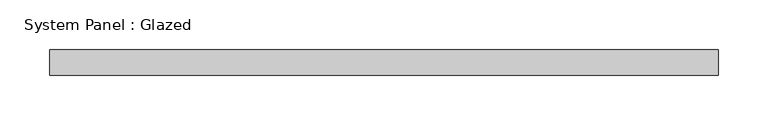
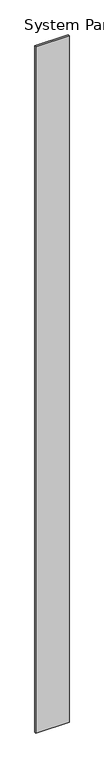
"""IFC4 building model written with IfcOpenShell, lengths in millimetres: plate geometry, System Panel : Glazed."""

from ifc_helpers import new_model, si_unit, origin, origin_with_axes, place, context, project, spatial, polyline, outline, extrude, source, transform, mapped, element, save


def system_panel_glazed_8086c5aa(model_context):
    return source(origin(), model_context, "Body", "SweptSolid", [
        extrude(outline(polyline([(334.16875, 19.05), (-334.16875, 19.05), (-334.16875, 44.45), (334.16875, 44.45), (334.16875, 19.05)])), origin_with_axes(), (0.0, 0.0, 1.0), 14503.4),
    ])


if __name__ == "__main__":
    model = new_model("IFC4")
    model_context = context("Model", 3, world=origin())
    ifc_project = project(units=[si_unit("LENGTHUNIT", "METRE", prefix="MILLI")], contexts=[model_context])
    site = spatial("IfcSite", under=ifc_project)
    building = spatial("IfcBuilding", under=site)
    placement = place(None, origin())
    system_panel_glazed_shape = system_panel_glazed_8086c5aa(model_context)
    element("IfcPlate", 1, ObjectType="System Panel : Glazed", at=placement, inside=building, context=model_context, shape_type="MappedRepresentation", body=[
        mapped(system_panel_glazed_shape, transform((0.0, 0.0, 0.0), x_axis=(1.0, 0.0, 0.0), y_axis=(0.0, 1.0, 0.0), z_axis=(0.0, 0.0, 1.0))),
    ])
    save(model, "model.ifc")

# Revit data of these elements
# Type "System Panel : Glazed"
#   Construction Type Id = "GSP4R"
#   Analytic Construction = "1/8 in Pilkington single glazing"
#   Visual Light Transmittance = 0.9
#   Solar Heat Gain Coefficient = 0.86
#   Heat Transfer Coefficient (U) = 1.18115 BTU/(h·ft²·°F)
# Element 1 (IfcPlate, "System Panel : Glazed")
#   Materials on its faces: "Glass"
# Materials
#   "Glass": class "Glass", colour RGB 0 128 192, transparency 0.75, Description = "Soda Lime Glass", Cost = 0
